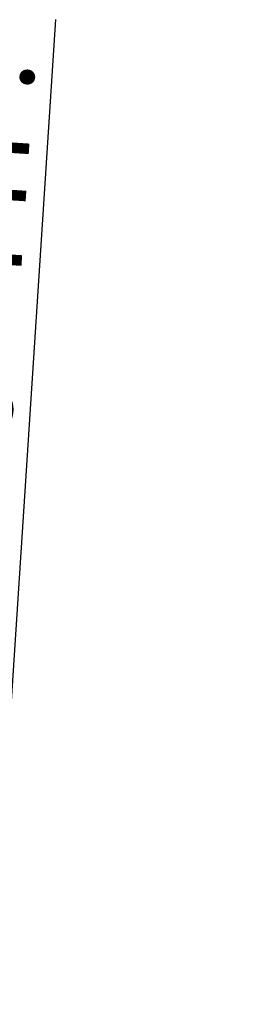
# Model space of a CAD drawing. Units: inches. Extents: x 3064 to 19385, y 846 to 15425.
# Tile 80 of 108: x 6629 to 6652, y 2013 to 2118. Entities that reach past the tile are written whole.
import ezdxf

# ---------------------------------------------------------------- set-up
doc = ezdxf.new("R2010")
doc.units = ezdxf.units.IN
doc.layers.add('A-ANNO-DIMS', color=2, linetype='Continuous', lineweight=18)
doc.styles.get("Standard").update_dxf_attribs({"font": 'arial.ttf'})
doc.dimstyles.new('ISO-25', dxfattribs={"dimtxt": 9, "dimasz": 2.5, "dimexe": 1.25, "dimexo": 0.625, "dimtad": 1, "dimdec": 1, "dimlunit": 3, "dimtxsty": 'Standard', "dimcen": 2.5, "dimadec": 0, "dimazin": 0, "dimtfac": 1, "dimtdec": 1, "dimtmove": 0, "dimatfit": 3, "dimfxl": 1, "dimarcsym": 0})

# ---------------------------------------------------------------- blocks, each defined once
blk = doc.blocks.new('*D433')
at = {"layer": 'A-ANNO-DIMS', "color": 0, "lineweight": -2, "transparency": 16777216}
for p, q in [((6621.84, 1945.07), (6633.12, 2118.25)), ((6612.14, 1945.71), (6623.09, 1944.99)), ((6617.52, 1878.71), (6621.68, 1942.58)), ((6607.65, 1876.85), (6618.61, 1876.14))]:
    blk.add_line(p, q, dxfattribs=at)
at = {"layer": 'A-ANNO-DIMS', "color": 0, "transparency": 16777216}
for points in [[(6621.26, 1942.61), (6622.09, 1942.55), (6621.84, 1945.07)], [(6617.11, 1878.74), (6617.94, 1878.69), (6617.36, 1876.22)]]:
    blk.add_solid(points, dxfattribs=at)
at = {"layer": 'Defpoints', "color": 0, "transparency": 16777216}
for p in [(6611.51, 1945.75), (6621.84, 1945.07), (6607.03, 1876.89)]:
    blk.add_point(p, dxfattribs=at)
at = {"layer": 'A-ANNO-DIMS', "color": 0, "transparency": 16777216, "insert": (6622.29, 2033.25), "char_height": 9, "attachment_point": 5, "rotation": 86.2748}
blk.add_mtext('WINDOW W1900-A 5\'-9" TYP.', dxfattribs=at)

msp = doc.modelspace()

# ---------------------------------------------------------------- dimensions: what is measured, and where the dimension line sits
at = {"layer": 'A-ANNO-DIMS'}
dim = msp.add_linear_dim(base=(6621.84, 1945.07), p1=(6607.03, 1876.89), p2=(6611.51, 1945.75), angle=86.2748, text='WINDOW W1900-A <> TYP.', dimstyle='ISO-25', override={"dimdec": 1, "dimrnd": 0, "dimzin": 1, "dimlunit": 4, "dimfrac": 2}, dxfattribs=at)
dim.commit()
dim.dimension.update_dxf_attribs({"geometry": '*D433', "text_midpoint": (6622.29, 2033.25)})

doc.saveas('drawing.dxf')
